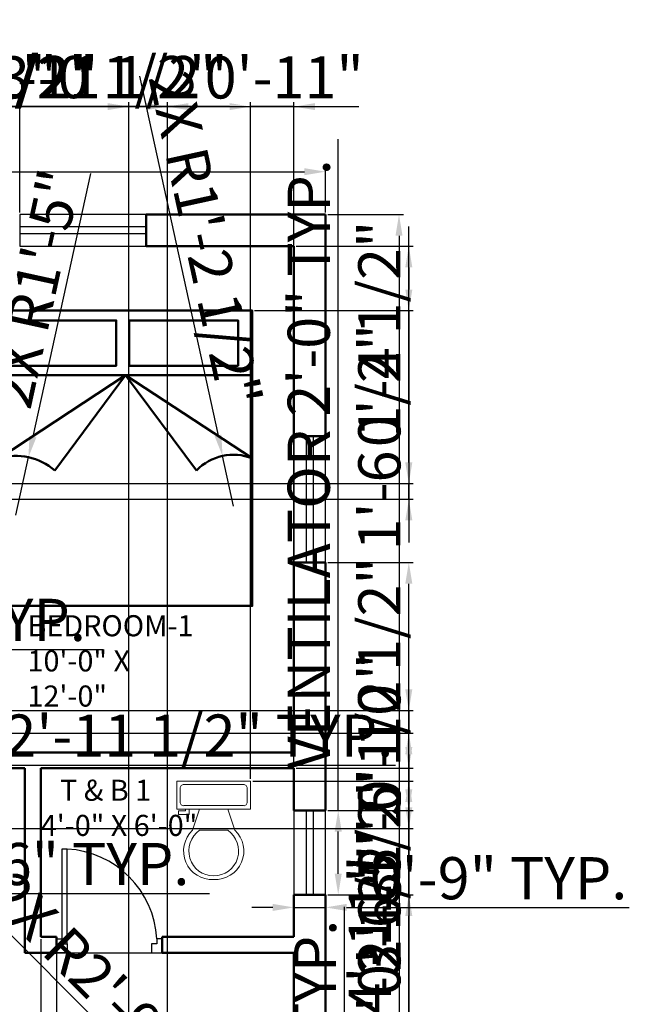
# Model space of a CAD drawing. Units: inches. Extents: x 1086 to 1501, y 383 to 973.
# Tile 7 of 7: x 1316 to 1490, y 611 to 891. Entities that reach past the tile are written whole.
import ezdxf

# ---------------------------------------------------------------- set-up
doc = ezdxf.new("R2010")
doc.units = ezdxf.units.IN
for name, color, linetype, lineweight in [('A-ANNO-DIMS', 2, 'Continuous', 18), ('A-AREA-IDEN', 7, 'Continuous', 25), ('A-FLOR-FIXT', 9, 'Continuous', 18), ('door', 10, 'Continuous', 25), ('furniture', 255, 'Continuous', 18), ('ventilator', 151, 'Continuous', 25), ('wall', 7, 'Continuous', 50), ('window', 81, 'Continuous', 25)]:
    doc.layers.add(name, color=color, linetype=linetype, lineweight=lineweight)
doc.styles.get("Standard").update_dxf_attribs({"font": 'arial.ttf'})
doc.dimstyles.new('ISO-25', dxfattribs={"dimtxt": 12, "dimasz": 6, "dimexe": 1.25, "dimexo": 0.625, "dimtad": 1, "dimdec": 1, "dimlunit": 3, "dimtxsty": 'Standard', "dimcen": 2.5, "dimadec": 0, "dimazin": 0, "dimtfac": 1, "dimtdec": 1, "dimtmove": 0, "dimatfit": 3, "dimfxl": 1, "dimarcsym": 0})

# ---------------------------------------------------------------- blocks, each defined once
blk = doc.blocks.new('d1')
at = {"layer": 'door'}
blk.add_line((1603.89, 536.69), (1633.89, 536.69), dxfattribs=at)
blk.add_lwpolyline([(1605.39, 539.19), (1606.89, 539.19), (1606.89, 566.19), (1605.39, 566.19)], close=True, dxfattribs=at)
for points in [[(1606.89, 536.69), (1603.89, 536.69), (1603.89, 540.69), (1605.39, 540.69), (1605.39, 539.19), (1606.89, 539.19), (1606.89, 536.69)], [(1630.89, 536.69), (1633.89, 536.69), (1633.89, 540.69), (1632.39, 540.69), (1632.39, 539.19), (1630.89, 539.19), (1630.89, 536.69)]]:
    blk.add_lwpolyline(points, dxfattribs=at)
blk.add_arc((1605.39, 539.19), 27.04, 3.1798, 86.8202, dxfattribs=at)
blk = doc.blocks.new('v')
at = {"layer": 'ventilator'}
for p, q in [((1539.56, 920.22), (1539.56, 896.22)), ((1541.56, 920.22), (1541.56, 896.22))]:
    blk.add_line(p, q, dxfattribs=at)
blk.add_lwpolyline([(1536.06, 896.22), (1545.06, 896.22), (1545.06, 920.22), (1536.06, 920.22)], close=True, dxfattribs=at)
blk = doc.blocks.new('w1')
at = {"layer": 'window'}
for p, q in [((1475.33, 845.32), (1475.33, 809.32)), ((1477.33, 845.32), (1477.33, 809.32))]:
    blk.add_line(p, q, dxfattribs=at)
blk.add_lwpolyline([(1471.83, 809.32), (1480.83, 809.32), (1480.83, 845.32), (1471.83, 845.32)], close=True, dxfattribs=at)
blk = doc.blocks.new('bed')
at = {"layer": 'wall'}
for p, q in [((1549.71, 859.44), (1621.71, 859.44)), ((1585.71, 859.44), (1549.71, 835.76)), ((1585.71, 859.44), (1565.54, 832.3)), ((1585.71, 859.44), (1621.71, 835.76)), ((1585.71, 859.44), (1605.88, 832.3))]:
    blk.add_line(p, q, dxfattribs=at)
for points in [[(1549.71, 793.76), (1621.71, 793.76), (1621.71, 877.76), (1549.71, 877.76)], [(1552.04, 875), (1583.04, 875), (1583.04, 862.08), (1552.04, 862.08)], [(1586.71, 875), (1617.71, 875), (1617.71, 862.08), (1586.71, 862.08)]]:
    blk.add_lwpolyline(points, close=True, dxfattribs=at)
for centre, radius, start, end in [((1554.45, 819.53), 16.91, 49.0428, 106.2967), ((1616.39, 822.13), 14.63, 68.7093, 135.9513)]:
    blk.add_arc(centre, radius, start, end, dxfattribs=at)
blk = doc.blocks.new('*U8')
for p, q in [((241.3, -152.4), (241.3, -50.8)), ((-203.2, -215.9), (-203.2, -203.2)), ((-177.8, -203.2), (-177.8, -241.3)), ((-101.6, -203.2), (-152.4, -355.6)), ((101.6, -203.2), (152.4, -355.6)), ((-254, -215.9), (-203.2, -215.9)), ((-254, -241.3), (-254, -215.9)), ((-177.8, -241.3), (-254, -241.3)), ((101.6, -355.6), (-101.6, -355.6))]:
    blk.add_line(p, q)
blk.add_lwpolyline([(266.7, -203.2), (266.7, 0), (-266.7, 0), (-266.7, -203.2)], close=True)
for points in [[(-241.3, -50.8), (-241.3, -152.4)], [(215.9, -25.4), (-215.9, -25.4)], [(-215.9, -177.8), (215.9, -177.8)]]:
    blk.add_lwpolyline(points)
for centre, radius, start, end in [((-219.075, -47.625), 22.45064, 81.8699, 188.1301), ((219.075, -47.625), 22.45064, 351.8699, 98.1301), ((-219.075, -155.575), 22.45064, 171.869898, 278.1301), ((219.075, -155.575), 22.45064, 261.8699, 8.1301), ((-12.12088, -505.93752), 205.61935, 133.01722, 273.38), ((0.94996, -504.77674), 181.02486, 124.50543, 269.7), ((-0.94742, -504.77674), 181.02486, 270.3, 55.4946), ((12.12342, -505.93752), 205.61935, 266.62, 46.9828)]:
    blk.add_arc(centre, radius, start, end)
blk = doc.blocks.new('*D9')
at = {"layer": 'A-ANNO-DIMS', "color": 0, "lineweight": -2, "transparency": 16777216}
for p, q in [((1133.43, 835.83), (1133.43, 848.67)), ((1139.43, 847.42), (1397.43, 847.42)), ((1403.43, 835.83), (1403.43, 848.67))]:
    blk.add_line(p, q, dxfattribs=at)
at = {"layer": 'A-ANNO-DIMS', "color": 0, "transparency": 16777216}
for points in [[(1139.43, 848.42), (1139.43, 846.42), (1133.43, 847.42)], [(1397.43, 848.42), (1397.43, 846.42), (1403.43, 847.42)]]:
    blk.add_solid(points, dxfattribs=at)
at = {"layer": 'Defpoints', "color": 0, "transparency": 16777216}
for p in [(1403.43, 847.42), (1133.43, 835.21), (1403.43, 835.21)]:
    blk.add_point(p, dxfattribs=at)
at = {"layer": 'A-ANNO-DIMS', "color": 0, "transparency": 16777216, "insert": (1268.43, 854.18), "char_height": 12, "attachment_point": 5}
blk.add_mtext('22\'-6"', dxfattribs=at)
blk = doc.blocks.new('*D10')
at = {"layer": 'A-ANNO-DIMS', "color": 0, "lineweight": -2, "transparency": 16777216}
for p, q in [((1404.05, 835.21), (1425.57, 835.21)), ((1424.32, 829.21), (1424.32, 422.21)), ((1404.05, 416.21), (1425.57, 416.21))]:
    blk.add_line(p, q, dxfattribs=at)
at = {"layer": 'A-ANNO-DIMS', "color": 0, "transparency": 16777216}
for points in [[(1423.32, 829.21), (1425.32, 829.21), (1424.32, 835.21)], [(1423.32, 422.21), (1425.32, 422.21), (1424.32, 416.21)]]:
    blk.add_solid(points, dxfattribs=at)
at = {"layer": 'Defpoints', "color": 0, "transparency": 16777216}
for p in [(1403.43, 835.21), (1403.43, 416.21), (1424.32, 416.21)]:
    blk.add_point(p, dxfattribs=at)
at = {"layer": 'A-ANNO-DIMS', "color": 0, "transparency": 16777216, "insert": (1417.56, 625.71), "char_height": 12, "attachment_point": 5, "rotation": 90}
blk.add_mtext('34\'-11"', dxfattribs=at)
blk = doc.blocks.new('*D13')
at = {"layer": 'A-ANNO-DIMS', "color": 0, "lineweight": -2, "transparency": 16777216}
for p, q in [((1408.83, 479.21), (1408.83, 638.31)), ((1404.05, 479.21), (1410.08, 479.21)), ((1408.83, 449.21), (1408.83, 473.21)), ((1404.05, 443.21), (1410.08, 443.21))]:
    blk.add_line(p, q, dxfattribs=at)
at = {"layer": 'A-ANNO-DIMS', "color": 0, "transparency": 16777216}
for points in [[(1407.83, 473.21), (1409.83, 473.21), (1408.83, 479.21)], [(1407.83, 449.21), (1409.83, 449.21), (1408.83, 443.21)]]:
    blk.add_solid(points, dxfattribs=at)
at = {"layer": 'Defpoints', "color": 0, "transparency": 16777216}
for p in [(1403.43, 479.21), (1408.83, 479.21), (1403.43, 443.21)]:
    blk.add_point(p, dxfattribs=at)
at = {"layer": 'A-ANNO-DIMS', "color": 0, "transparency": 16777216, "insert": (1401.99, 561.76), "char_height": 12, "attachment_point": 5, "rotation": 90}
blk.add_mtext('WINDOW 3\'-0" TYP.', dxfattribs=at)
blk = doc.blocks.new('*D15')
at = {"layer": 'A-ANNO-DIMS', "color": 0, "lineweight": -2, "transparency": 16777216}
for p, q in [((1407.03, 665.71), (1407.03, 856.64)), ((1404.05, 665.71), (1408.28, 665.71)), ((1407.03, 647.71), (1407.03, 659.71)), ((1404.05, 641.71), (1408.28, 641.71))]:
    blk.add_line(p, q, dxfattribs=at)
at = {"layer": 'A-ANNO-DIMS', "color": 0, "transparency": 16777216}
for points in [[(1406.03, 659.71), (1408.03, 659.71), (1407.03, 665.71)], [(1406.03, 647.71), (1408.03, 647.71), (1407.03, 641.71)]]:
    blk.add_solid(points, dxfattribs=at)
at = {"layer": 'Defpoints', "color": 0, "transparency": 16777216}
for p in [(1403.43, 665.71), (1407.03, 665.71), (1403.43, 641.71)]:
    blk.add_point(p, dxfattribs=at)
at = {"layer": 'A-ANNO-DIMS', "color": 0, "transparency": 16777216, "insert": (1400.2, 764.17), "char_height": 12, "attachment_point": 5, "rotation": 90}
blk.add_mtext('VENTILATOR 2\'-0" TYP.', dxfattribs=at)
blk = doc.blocks.new('*D16')
at = {"layer": 'A-ANNO-DIMS', "color": 0, "lineweight": -2, "transparency": 16777216}
for p, q in [((1394.43, 641.08), (1394.43, 636.86)), ((1403.43, 641.08), (1403.43, 636.86)), ((1388.43, 638.11), (1382.43, 638.11)), ((1394.43, 638.11), (1403.43, 638.11)), ((1409.43, 638.11), (1489.83, 638.11))]:
    blk.add_line(p, q, dxfattribs=at)
at = {"layer": 'A-ANNO-DIMS', "color": 0, "transparency": 16777216}
for points in [[(1388.43, 639.11), (1388.43, 637.11), (1394.43, 638.11)], [(1409.43, 639.11), (1409.43, 637.11), (1403.43, 638.11)]]:
    blk.add_solid(points, dxfattribs=at)
at = {"layer": 'Defpoints', "color": 0, "transparency": 16777216}
for p in [(1394.43, 641.71), (1403.43, 641.71), (1403.43, 638.11)]:
    blk.add_point(p, dxfattribs=at)
at = {"layer": 'A-ANNO-DIMS', "color": 0, "transparency": 16777216, "insert": (1452.63, 644.86), "char_height": 12, "attachment_point": 5}
blk.add_mtext('0\'-9" TYP.', dxfattribs=at)
blk = doc.blocks.new('*D19')
at = {"layer": 'A-ANNO-DIMS', "color": 0, "lineweight": -2, "transparency": 16777216}
for p, q in [((1306.05, 673.21), (1312.08, 673.21)), ((1310.83, 667.21), (1310.83, 643.21)), ((1306.05, 637.21), (1312.08, 637.21)), ((1310.83, 637.21), (1310.83, 411.12))]:
    blk.add_line(p, q, dxfattribs=at)
at = {"layer": 'A-ANNO-DIMS', "color": 0, "transparency": 16777216}
for points in [[(1309.83, 667.21), (1311.83, 667.21), (1310.83, 673.21)], [(1309.83, 643.21), (1311.83, 643.21), (1310.83, 637.21)]]:
    blk.add_solid(points, dxfattribs=at)
at = {"layer": 'Defpoints', "color": 0, "transparency": 16777216}
for p in [(1305.43, 673.21), (1305.43, 637.21), (1310.83, 637.21)]:
    blk.add_point(p, dxfattribs=at)
at = {"layer": 'A-ANNO-DIMS', "color": 0, "transparency": 16777216, "insert": (1303.99, 521.16), "char_height": 12, "attachment_point": 5, "rotation": 90}
blk.add_mtext('BEDROOM DOOR 3\'-0" TYP.', dxfattribs=at)
blk = doc.blocks.new('*D20')
at = {"layer": 'A-ANNO-DIMS', "color": 0, "lineweight": -2, "transparency": 16777216}
for p, q in [((1269.93, 673.83), (1269.93, 679.86)), ((1275.93, 678.61), (1299.43, 678.61)), ((1305.43, 673.83), (1305.43, 679.86)), ((1305.43, 678.61), (1423.32, 678.61))]:
    blk.add_line(p, q, dxfattribs=at)
at = {"layer": 'A-ANNO-DIMS', "color": 0, "transparency": 16777216}
for points in [[(1275.93, 679.61), (1275.93, 677.61), (1269.93, 678.61)], [(1299.43, 679.61), (1299.43, 677.61), (1305.43, 678.61)]]:
    blk.add_solid(points, dxfattribs=at)
at = {"layer": 'Defpoints', "color": 0, "transparency": 16777216}
for p in [(1305.43, 678.61), (1269.93, 673.21), (1305.43, 673.21)]:
    blk.add_point(p, dxfattribs=at)
at = {"layer": 'A-ANNO-DIMS', "color": 0, "transparency": 16777216, "insert": (1367.37, 685.44), "char_height": 12, "attachment_point": 5}
blk.add_mtext('2\'-11 1/2" TYP.', dxfattribs=at)
blk = doc.blocks.new('*D25')
at = {"layer": 'A-ANNO-DIMS', "color": 0, "lineweight": -2, "transparency": 16777216}
for p, q in [((1147.7, 709.78), (1147.7, 712.78)), ((1153.7, 711.53), (1157.51, 711.53)), ((1163.51, 709.78), (1163.51, 712.78)), ((1163.51, 711.53), (1340.15, 711.53))]:
    blk.add_line(p, q, dxfattribs=at)
at = {"layer": 'A-ANNO-DIMS', "color": 0, "transparency": 16777216}
for points in [[(1153.7, 712.53), (1153.7, 710.53), (1147.7, 711.53)], [(1157.51, 712.53), (1157.51, 710.53), (1163.51, 711.53)]]:
    blk.add_solid(points, dxfattribs=at)
at = {"layer": 'Defpoints', "color": 0, "transparency": 16777216}
for p in [(1163.51, 711.53), (1147.7, 709.16), (1163.51, 709.16)]:
    blk.add_point(p, dxfattribs=at)
at = {"layer": 'A-ANNO-DIMS', "color": 0, "transparency": 16777216, "insert": (1254.83, 718.36), "char_height": 12, "attachment_point": 5}
blk.add_mtext('END CHAIR 1\'-4" TYP.', dxfattribs=at)
blk = doc.blocks.new('*D27')
at = {"layer": 'A-ANNO-DIMS', "color": 0, "lineweight": -2, "transparency": 16777216}
for p, q in [((1171.32, 644.17), (1171.32, 640.82)), ((1177.32, 642.07), (1183.45, 642.07)), ((1189.45, 644.17), (1189.45, 640.82)), ((1189.45, 642.07), (1370.39, 642.07))]:
    blk.add_line(p, q, dxfattribs=at)
at = {"layer": 'A-ANNO-DIMS', "color": 0, "transparency": 16777216}
for points in [[(1177.32, 643.07), (1177.32, 641.07), (1171.32, 642.07)], [(1183.45, 643.07), (1183.45, 641.07), (1189.45, 642.07)]]:
    blk.add_solid(points, dxfattribs=at)
at = {"layer": 'Defpoints', "color": 0, "transparency": 16777216}
for p in [(1171.32, 644.79), (1189.45, 644.79), (1189.45, 642.07)]:
    blk.add_point(p, dxfattribs=at)
at = {"layer": 'A-ANNO-DIMS', "color": 0, "transparency": 16777216, "insert": (1282.92, 648.9), "char_height": 12, "attachment_point": 5}
blk.add_mtext('SIDE CHAIR 1\'-6" TYP.', dxfattribs=at)
blk = doc.blocks.new('*D31')
at = {"layer": 'A-ANNO-DIMS', "color": 0, "lineweight": -2, "transparency": 16777216}
for p, q in [((1256.43, 835.83), (1256.43, 867.19)), ((1262.43, 865.94), (1310.43, 865.94)), ((1316.43, 835.83), (1316.43, 867.19))]:
    blk.add_line(p, q, dxfattribs=at)
at = {"layer": 'A-ANNO-DIMS', "color": 0, "transparency": 16777216}
for points in [[(1262.43, 866.94), (1262.43, 864.94), (1256.43, 865.94)], [(1310.43, 866.94), (1310.43, 864.94), (1316.43, 865.94)]]:
    blk.add_solid(points, dxfattribs=at)
at = {"layer": 'Defpoints', "color": 0, "transparency": 16777216}
for p in [(1316.43, 865.94), (1256.43, 835.21), (1316.43, 835.21)]:
    blk.add_point(p, dxfattribs=at)
at = {"layer": 'A-ANNO-DIMS', "color": 0, "transparency": 16777216, "insert": (1286.43, 872.69), "char_height": 12, "attachment_point": 5}
blk.add_mtext('5\'-0"', dxfattribs=at)
blk = doc.blocks.new('*D36')
at = {"layer": 'A-ANNO-DIMS', "color": 0, "lineweight": -2, "transparency": 16777216}
for p, q in [((1427.11, 641.71), (1427.11, 708.82)), ((1404.05, 641.71), (1428.36, 641.71)), ((1427.11, 587.46), (1427.11, 635.71)), ((1404.05, 581.46), (1428.36, 581.46))]:
    blk.add_line(p, q, dxfattribs=at)
at = {"layer": 'A-ANNO-DIMS', "color": 0, "transparency": 16777216}
for points in [[(1426.11, 635.71), (1428.11, 635.71), (1427.11, 641.71)], [(1426.11, 587.46), (1428.11, 587.46), (1427.11, 581.46)]]:
    blk.add_solid(points, dxfattribs=at)
at = {"layer": 'Defpoints', "color": 0, "transparency": 16777216}
for p in [(1403.43, 641.71), (1427.11, 641.71), (1403.43, 581.46)]:
    blk.add_point(p, dxfattribs=at)
at = {"layer": 'A-ANNO-DIMS', "color": 0, "transparency": 16777216, "insert": (1420.28, 678.26), "char_height": 12, "attachment_point": 5, "rotation": 90}
blk.add_mtext('5\'-0 1/2"', dxfattribs=at)
blk = doc.blocks.new('*D37')
at = {"layer": 'A-ANNO-DIMS', "color": 0, "lineweight": -2, "transparency": 16777216}
for p, q in [((1404.05, 736.21), (1428.36, 736.21)), ((1427.11, 671.71), (1427.11, 730.21)), ((1404.05, 665.71), (1428.36, 665.71))]:
    blk.add_line(p, q, dxfattribs=at)
at = {"layer": 'A-ANNO-DIMS', "color": 0, "transparency": 16777216}
for points in [[(1426.11, 730.21), (1428.11, 730.21), (1427.11, 736.21)], [(1426.11, 671.71), (1428.11, 671.71), (1427.11, 665.71)]]:
    blk.add_solid(points, dxfattribs=at)
at = {"layer": 'Defpoints', "color": 0, "transparency": 16777216}
for p in [(1403.43, 736.21), (1427.11, 736.21), (1403.43, 665.71)]:
    blk.add_point(p, dxfattribs=at)
at = {"layer": 'A-ANNO-DIMS', "color": 0, "transparency": 16777216, "insert": (1420.28, 700.96), "char_height": 12, "attachment_point": 5, "rotation": 90}
blk.add_mtext('5\'-10 1/2"', dxfattribs=at)
blk = doc.blocks.new('*D42')
at = {"layer": 'A-ANNO-DIMS', "color": 0, "lineweight": -2, "transparency": 16777216}
for p, q in [((1256.43, 502.33), (1256.43, 867.19)), ((1262.43, 865.94), (1263.93, 865.94)), ((1269.93, 502.33), (1269.93, 867.19)), ((1269.93, 865.94), (1335.91, 865.94))]:
    blk.add_line(p, q, dxfattribs=at)
at = {"layer": 'A-ANNO-DIMS', "color": 0, "transparency": 16777216}
for points in [[(1262.43, 866.94), (1262.43, 864.94), (1256.43, 865.94)], [(1263.93, 866.94), (1263.93, 864.94), (1269.93, 865.94)]]:
    blk.add_solid(points, dxfattribs=at)
at = {"layer": 'Defpoints', "color": 0, "transparency": 16777216}
for p in [(1269.93, 865.94), (1256.43, 501.71), (1269.93, 501.71)]:
    blk.add_point(p, dxfattribs=at)
at = {"layer": 'A-ANNO-DIMS', "color": 0, "transparency": 16777216, "insert": (1305.92, 872.77), "char_height": 12, "attachment_point": 5}
blk.add_mtext('1\'-1 1/2"', dxfattribs=at)
blk = doc.blocks.new('*D45')
at = {"layer": 'A-ANNO-DIMS', "color": 0, "lineweight": -2, "transparency": 16777216}
for p, q in [((1259.43, 497.83), (1259.43, 867.19)), ((1265.43, 865.94), (1352.43, 865.94)), ((1358.43, 497.83), (1358.43, 867.19))]:
    blk.add_line(p, q, dxfattribs=at)
at = {"layer": 'A-ANNO-DIMS', "color": 0, "transparency": 16777216}
for points in [[(1265.43, 866.94), (1265.43, 864.94), (1259.43, 865.94)], [(1352.43, 866.94), (1352.43, 864.94), (1358.43, 865.94)]]:
    blk.add_solid(points, dxfattribs=at)
at = {"layer": 'Defpoints', "color": 0, "transparency": 16777216}
for p in [(1358.43, 865.94), (1259.43, 497.21), (1358.43, 497.21)]:
    blk.add_point(p, dxfattribs=at)
at = {"layer": 'A-ANNO-DIMS', "color": 0, "transparency": 16777216, "insert": (1308.93, 872.7), "char_height": 12, "attachment_point": 5}
blk.add_mtext('8\'-3"', dxfattribs=at)
blk = doc.blocks.new('*D47')
at = {"layer": 'A-ANNO-DIMS', "color": 0, "lineweight": -2, "transparency": 16777216}
for p, q in [((1341.43, 865.94), (1335.43, 865.94)), ((1347.43, 425.83), (1347.43, 867.19)), ((1347.43, 865.94), (1358.43, 865.94)), ((1358.43, 425.83), (1358.43, 867.19)), ((1364.43, 865.94), (1412.9, 865.94))]:
    blk.add_line(p, q, dxfattribs=at)
at = {"layer": 'A-ANNO-DIMS', "color": 0, "transparency": 16777216}
for points in [[(1341.43, 866.94), (1341.43, 864.94), (1347.43, 865.94)], [(1364.43, 866.94), (1364.43, 864.94), (1358.43, 865.94)]]:
    blk.add_solid(points, dxfattribs=at)
at = {"layer": 'Defpoints', "color": 0, "transparency": 16777216}
for p in [(1358.43, 865.94), (1347.43, 425.21), (1358.43, 425.21)]:
    blk.add_point(p, dxfattribs=at)
at = {"layer": 'A-ANNO-DIMS', "color": 0, "transparency": 16777216, "insert": (1391.67, 872.69), "char_height": 12, "attachment_point": 5}
blk.add_mtext('0\'-11"', dxfattribs=at)
blk = doc.blocks.new('*D54')
at = {"layer": 'A-ANNO-DIMS', "color": 0, "lineweight": -2, "transparency": 16777216}
for p, q in [((1427.11, 764.71), (1427.11, 831.82)), ((1270.55, 758.71), (1428.36, 758.71)), ((1427.11, 754.21), (1427.11, 758.71)), ((1270.55, 754.21), (1428.36, 754.21)), ((1427.11, 748.21), (1427.11, 742.21))]:
    blk.add_line(p, q, dxfattribs=at)
at = {"layer": 'A-ANNO-DIMS', "color": 0, "transparency": 16777216}
for points in [[(1426.11, 764.71), (1428.11, 764.71), (1427.11, 758.71)], [(1426.11, 748.21), (1428.11, 748.21), (1427.11, 754.21)]]:
    blk.add_solid(points, dxfattribs=at)
at = {"layer": 'Defpoints', "color": 0, "transparency": 16777216}
for p in [(1269.93, 758.71), (1427.11, 758.71), (1269.93, 754.21)]:
    blk.add_point(p, dxfattribs=at)
at = {"layer": 'A-ANNO-DIMS', "color": 0, "transparency": 16777216, "insert": (1420.28, 801.26), "char_height": 12, "attachment_point": 5, "rotation": 90}
blk.add_mtext('0\'-4 1/2"', dxfattribs=at)
blk = doc.blocks.new('*D60')
at = {"layer": 'A-ANNO-DIMS', "color": 0, "lineweight": -2, "transparency": 16777216}
for p, q in [((1322.43, 629.08), (1322.43, 392.46)), ((1326.93, 629.08), (1326.93, 392.46)), ((1316.43, 393.71), (1310.43, 393.71)), ((1322.43, 393.71), (1326.93, 393.71)), ((1332.93, 393.71), (1400.04, 393.71))]:
    blk.add_line(p, q, dxfattribs=at)
at = {"layer": 'A-ANNO-DIMS', "color": 0, "transparency": 16777216}
for points in [[(1316.43, 394.71), (1316.43, 392.71), (1322.43, 393.71)], [(1332.93, 394.71), (1332.93, 392.71), (1326.93, 393.71)]]:
    blk.add_solid(points, dxfattribs=at)
at = {"layer": 'Defpoints', "color": 0, "transparency": 16777216}
for p in [(1322.43, 629.71), (1326.93, 629.71), (1326.93, 393.71)]:
    blk.add_point(p, dxfattribs=at)
at = {"layer": 'A-ANNO-DIMS', "color": 0, "transparency": 16777216, "insert": (1369.49, 400.54), "char_height": 12, "attachment_point": 5}
blk.add_mtext('0\'-4 1/2"', dxfattribs=at)
blk = doc.blocks.new('*D61')
at = {"layer": 'A-ANNO-DIMS', "color": 0, "lineweight": -2, "transparency": 16777216}
for p, q in [((1376.11, 865.94), (1310.13, 865.94)), ((1382.11, 674.69), (1382.11, 867.19)), ((1394.43, 865.94), (1382.11, 865.94)), ((1394.43, 678.33), (1394.43, 867.19)), ((1400.43, 865.94), (1406.43, 865.94))]:
    blk.add_line(p, q, dxfattribs=at)
at = {"layer": 'A-ANNO-DIMS', "color": 0, "transparency": 16777216}
for points in [[(1376.11, 866.94), (1376.11, 864.94), (1382.11, 865.94)], [(1400.43, 866.94), (1400.43, 864.94), (1394.43, 865.94)]]:
    blk.add_solid(points, dxfattribs=at)
at = {"layer": 'Defpoints', "color": 0, "transparency": 16777216}
for p in [(1382.11, 865.94), (1394.43, 677.71), (1382.11, 674.06)]:
    blk.add_point(p, dxfattribs=at)
at = {"layer": 'A-ANNO-DIMS', "color": 0, "transparency": 16777216, "insert": (1340.12, 872.77), "char_height": 12, "attachment_point": 5}
blk.add_mtext('1\'-0 1/2"', dxfattribs=at)
blk = doc.blocks.new('*D62')
at = {"layer": 'A-ANNO-DIMS', "color": 0, "lineweight": -2, "transparency": 16777216}
for p, q in [((1427.11, 683.71), (1427.11, 689.71)), ((1395.05, 677.71), (1428.36, 677.71)), ((1427.11, 677.71), (1427.11, 674.06)), ((1382.74, 674.06), (1428.36, 674.06)), ((1427.11, 668.06), (1427.11, 600.95))]:
    blk.add_line(p, q, dxfattribs=at)
at = {"layer": 'A-ANNO-DIMS', "color": 0, "transparency": 16777216}
for points in [[(1426.11, 683.71), (1428.11, 683.71), (1427.11, 677.71)], [(1426.11, 668.06), (1428.11, 668.06), (1427.11, 674.06)]]:
    blk.add_solid(points, dxfattribs=at)
at = {"layer": 'Defpoints', "color": 0, "transparency": 16777216}
for p in [(1394.43, 677.71), (1382.11, 674.06), (1427.11, 674.06)]:
    blk.add_point(p, dxfattribs=at)
at = {"layer": 'A-ANNO-DIMS', "color": 0, "transparency": 16777216, "insert": (1420.28, 631.51), "char_height": 12, "attachment_point": 5, "rotation": 90}
blk.add_mtext('0\'-3 1/2"', dxfattribs=at)
blk = doc.blocks.new('*D66')
at = {"layer": 'A-ANNO-DIMS', "color": 0, "lineweight": -2, "transparency": 16777216}
for p, q in [((1190.08, 687.66), (1428.36, 687.66)), ((1427.11, 681.66), (1427.11, 666.6)), ((1190.08, 660.6), (1428.36, 660.6)), ((1427.11, 660.6), (1427.11, 621.25))]:
    blk.add_line(p, q, dxfattribs=at)
at = {"layer": 'A-ANNO-DIMS', "color": 0, "transparency": 16777216}
for points in [[(1426.11, 681.66), (1428.11, 681.66), (1427.11, 687.66)], [(1426.11, 666.6), (1428.11, 666.6), (1427.11, 660.6)]]:
    blk.add_solid(points, dxfattribs=at)
at = {"layer": 'Defpoints', "color": 0, "transparency": 16777216}
for p in [(1189.45, 687.66), (1189.45, 660.6), (1427.11, 660.6)]:
    blk.add_point(p, dxfattribs=at)
at = {"layer": 'A-ANNO-DIMS', "color": 0, "transparency": 16777216, "insert": (1420.36, 637.93), "char_height": 12, "attachment_point": 5, "rotation": 90}
blk.add_mtext('2\'-3"', dxfattribs=at)
blk = doc.blocks.new('*D67')
at = {"layer": 'A-ANNO-DIMS', "color": 0, "lineweight": -2, "transparency": 16777216}
for p, q in [((1427.11, 700.13), (1427.11, 706.13)), ((1171.95, 694.13), (1428.36, 694.13)), ((1427.11, 694.13), (1427.11, 687.66)), ((1190.08, 687.66), (1428.36, 687.66)), ((1427.11, 681.66), (1427.11, 614.55))]:
    blk.add_line(p, q, dxfattribs=at)
at = {"layer": 'A-ANNO-DIMS', "color": 0, "transparency": 16777216}
for points in [[(1426.11, 700.13), (1428.11, 700.13), (1427.11, 694.13)], [(1426.11, 681.66), (1428.11, 681.66), (1427.11, 687.66)]]:
    blk.add_solid(points, dxfattribs=at)
at = {"layer": 'Defpoints', "color": 0, "transparency": 16777216}
for p in [(1171.32, 694.13), (1189.45, 687.66), (1427.11, 687.66)]:
    blk.add_point(p, dxfattribs=at)
at = {"layer": 'A-ANNO-DIMS', "color": 0, "transparency": 16777216, "insert": (1420.28, 645.1), "char_height": 12, "attachment_point": 5, "rotation": 90}
blk.add_mtext('0\'-6 1/2"', dxfattribs=at)
blk = doc.blocks.new('*D69')
at = {"layer": 'A-ANNO-DIMS', "color": 0, "lineweight": -2, "transparency": 16777216}
for p, q in [((1236.63, 603.21), (1236.63, 867.19)), ((1242.63, 865.94), (1263.93, 865.94)), ((1269.93, 603.25), (1269.93, 867.19)), ((1269.93, 865.94), (1337.25, 865.94))]:
    blk.add_line(p, q, dxfattribs=at)
at = {"layer": 'A-ANNO-DIMS', "color": 0, "transparency": 16777216}
for points in [[(1242.63, 866.94), (1242.63, 864.94), (1236.63, 865.94)], [(1263.93, 866.94), (1263.93, 864.94), (1269.93, 865.94)]]:
    blk.add_solid(points, dxfattribs=at)
at = {"layer": 'Defpoints', "color": 0, "transparency": 16777216}
for p in [(1269.93, 865.94), (1236.63, 602.59), (1269.93, 602.62)]:
    blk.add_point(p, dxfattribs=at)
at = {"layer": 'A-ANNO-DIMS', "color": 0, "transparency": 16777216, "insert": (1306.59, 872.77), "char_height": 12, "attachment_point": 5}
blk.add_mtext('2\'-9 1/2"', dxfattribs=at)
blk = doc.blocks.new('*D74')
at = {"layer": 'A-ANNO-DIMS', "color": 0, "lineweight": -2, "transparency": 16777216}
for p, q in [((1395.05, 826.21), (1428.36, 826.21)), ((1427.11, 820.21), (1427.11, 813.89)), ((1383.18, 807.89), (1428.36, 807.89)), ((1427.11, 807.89), (1427.11, 741.91))]:
    blk.add_line(p, q, dxfattribs=at)
at = {"layer": 'A-ANNO-DIMS', "color": 0, "transparency": 16777216}
for points in [[(1426.11, 820.21), (1428.11, 820.21), (1427.11, 826.21)], [(1426.11, 813.89), (1428.11, 813.89), (1427.11, 807.89)]]:
    blk.add_solid(points, dxfattribs=at)
at = {"layer": 'Defpoints', "color": 0, "transparency": 16777216}
for p in [(1394.43, 826.21), (1382.55, 807.89), (1427.11, 807.89)]:
    blk.add_point(p, dxfattribs=at)
at = {"layer": 'A-ANNO-DIMS', "color": 0, "transparency": 16777216, "insert": (1420.28, 771.9), "char_height": 12, "attachment_point": 5, "rotation": 90}
blk.add_mtext('1\'-6 1/2"', dxfattribs=at)
blk = doc.blocks.new('*D77')
at = {"layer": 'A-ANNO-DIMS', "color": 0, "lineweight": -2, "transparency": 16777216}
for p, q in [((1274.43, 502.33), (1274.43, 867.19)), ((1280.43, 865.94), (1292.14, 865.94)), ((1298.14, 513.04), (1298.14, 867.19)), ((1298.14, 865.94), (1373.44, 865.94))]:
    blk.add_line(p, q, dxfattribs=at)
at = {"layer": 'A-ANNO-DIMS', "color": 0, "transparency": 16777216}
for points in [[(1280.43, 866.94), (1280.43, 864.94), (1274.43, 865.94)], [(1292.14, 866.94), (1292.14, 864.94), (1298.14, 865.94)]]:
    blk.add_solid(points, dxfattribs=at)
at = {"layer": 'Defpoints', "color": 0, "transparency": 16777216}
for p in [(1298.14, 865.94), (1298.14, 512.42), (1274.43, 501.71)]:
    blk.add_point(p, dxfattribs=at)
at = {"layer": 'A-ANNO-DIMS', "color": 0, "transparency": 16777216, "insert": (1338.79, 872.77), "char_height": 12, "attachment_point": 5}
blk.add_mtext('1\'-11 1/2"', dxfattribs=at)
blk = doc.blocks.new('*D78')
at = {"layer": 'A-ANNO-DIMS', "color": 0, "lineweight": -2, "transparency": 16777216}
for p, q in [((1272.43, 671.71), (1295.79, 648.35)), ((1354.21, 589.92), (1300.03, 644.11))]:
    blk.add_line(p, q, dxfattribs=at)
at = {"layer": 'A-ANNO-DIMS', "color": 0, "transparency": 16777216}
blk.add_solid([(1300.74, 644.81), (1299.32, 643.4), (1295.79, 648.35)], dxfattribs=at)
at = {"layer": 'Defpoints', "color": 0, "transparency": 16777216}
for p in [(1272.43, 671.71), (1295.79, 648.35)]:
    blk.add_point(p, dxfattribs=at)
at = {"layer": 'A-ANNO-DIMS', "color": 0, "transparency": 16777216, "insert": (1334.02, 619.67), "char_height": 12, "attachment_point": 5, "rotation": 314.9994}
blk.add_mtext('2X R2\'-9"', dxfattribs=at)
blk = doc.blocks.new('*D81')
at = {"layer": 'A-ANNO-DIMS', "color": 0, "lineweight": -2, "transparency": 16777216}
for p, q in [((1336.56, 846.9), (1320.19, 772.04)), ((1315.3, 749.66), (1318.91, 766.18))]:
    blk.add_line(p, q, dxfattribs=at)
at = {"layer": 'A-ANNO-DIMS', "color": 0, "transparency": 16777216}
blk.add_solid([(1319.22, 772.25), (1321.17, 771.83), (1318.91, 766.18)], dxfattribs=at)
at = {"layer": 'Defpoints', "color": 0, "transparency": 16777216}
for p in [(1318.91, 766.18), (1315.3, 749.66)]:
    blk.add_point(p, dxfattribs=at)
at = {"layer": 'A-ANNO-DIMS', "color": 0, "transparency": 16777216, "insert": (1322.42, 813.84), "char_height": 12, "attachment_point": 5, "rotation": 77.6694}
blk.add_mtext('2X R1\'-5"', dxfattribs=at)
blk = doc.blocks.new('*D82')
at = {"layer": 'A-ANNO-DIMS', "color": 0, "lineweight": -2, "transparency": 16777216}
for p, q in [((1350.51, 874.58), (1372.84, 772.41)), ((1377.24, 752.26), (1374.12, 766.55))]:
    blk.add_line(p, q, dxfattribs=at)
at = {"layer": 'A-ANNO-DIMS', "color": 0, "transparency": 16777216}
blk.add_solid([(1373.81, 772.63), (1371.86, 772.2), (1374.12, 766.55)], dxfattribs=at)
at = {"layer": 'Defpoints', "color": 0, "transparency": 16777216}
for p in [(1374.12, 766.55), (1377.24, 752.26)]:
    blk.add_point(p, dxfattribs=at)
at = {"layer": 'A-ANNO-DIMS', "color": 0, "transparency": 16777216, "insert": (1367.7, 827.89), "char_height": 12, "attachment_point": 5, "rotation": 282.3285}
blk.add_mtext('2X R1\'-2 1/2"', dxfattribs=at)

msp = doc.modelspace()

# ---------------------------------------------------------------- linework, layer by layer
at = {"layer": 'wall'}
for p, q in [((1403.43, 835.21), (1352.43, 835.21)), ((1352.43, 826.21), (1352.43, 835.21)), ((1403.43, 772.21), (1403.43, 835.21)), ((1394.43, 826.21), (1352.43, 826.21)), ((1394.43, 772.21), (1394.43, 826.21)), ((1394.43, 772.21), (1403.43, 772.21)), ((1394.43, 682.21), (1394.43, 736.21)), ((1394.43, 736.21), (1403.43, 736.21)), ((1403.43, 665.71), (1403.43, 736.21)), ((1394.43, 682.21), (1274.43, 682.21)), ((1317.93, 677.71), (1274.43, 677.71)), ((1317.93, 625.21), (1317.93, 677.71)), ((1394.43, 677.71), (1322.43, 677.71)), ((1322.43, 629.71), (1322.43, 677.71)), ((1394.43, 665.71), (1394.43, 677.71)), ((1394.43, 665.71), (1403.43, 665.71)), ((1394.43, 629.71), (1394.43, 641.71)), ((1394.43, 641.71), (1403.43, 641.71)), ((1403.43, 581.46), (1403.43, 641.71)), ((1326.93, 629.71), (1322.43, 629.71)), ((1326.93, 625.21), (1326.93, 629.71)), ((1394.43, 629.71), (1356.93, 629.71)), ((1356.93, 625.21), (1356.93, 629.71)), ((1326.93, 625.21), (1317.93, 625.21)), ((1394.43, 625.21), (1356.93, 625.21)), ((1394.43, 581.46), (1394.43, 625.21))]:
    msp.add_line(p, q, dxfattribs=at)

# ---------------------------------------------------------------- block references
at = {"layer": 'A-FLOR-FIXT', "xscale": 0.0393700787401575, "yscale": 0.0393700787401575, "zscale": 0.0393700787401575}
msp.add_blockref('*U8', (1371.61, 674.06), dxfattribs=at)
at = {"layer": 'door'}
msp.add_blockref('d1', (-276.96, 88.52), dxfattribs=at)
at = {"layer": 'furniture'}
msp.add_blockref('bed', (-239.15, -69.87), dxfattribs=at)
at = {"layer": 'ventilator'}
msp.add_blockref('v', (-141.63, -254.51), dxfattribs=at)
at = {"layer": 'window', "rotation": 270}
msp.add_blockref('w1', (507.11, 2307.04), dxfattribs=at)
at = {"layer": 'window'}
msp.add_blockref('w1', (-77.4, -73.11), dxfattribs=at)

# ---------------------------------------------------------------- texts
at = {"layer": 'A-AREA-IDEN', "char_height": 6, "attachment_point": 1}
for s, insert in [('BEDROOM-1\\P10\'-0" X 12\'-0"', (1318.65, 721.25)), ('   T & B 1\\P4\'-0" X 6\'-0"', (1322.43, 674.45))]:
    msp.add_mtext_dynamic_manual_height_columns(s, width=53.2651, gutter_width=12.5, heights=[0], dxfattribs=dict(at, insert=insert))

# ---------------------------------------------------------------- dimensions: what is measured, and where the dimension line sits
at = {"layer": 'A-ANNO-DIMS'}
for base, p1, p2, override, picture, middle in [((1269.93, 865.94), (1236.63, 602.59), (1269.93, 602.62), {"dimdec": 1, "dimlfac": 1, "dimrnd": 0, "dimzin": 1, "dimdsep": 46, "dimlunit": 4, "dimfrac": 2}, '*D69', (1306.59, 872.77)), ((1269.93, 865.94), (1256.43, 501.71), (1269.93, 501.71), {"dimdec": 1, "dimlfac": 1, "dimrnd": 0, "dimzin": 1, "dimdsep": 46, "dimlunit": 4, "dimfrac": 2}, '*D42', (1305.92, 872.77)), ((1298.14, 865.94), (1274.43, 501.71), (1298.14, 512.42), {"dimdec": 1, "dimlfac": 1, "dimrnd": 0, "dimzin": 1, "dimdsep": 46, "dimlunit": 4, "dimfrac": 2}, '*D77', (1338.79, 872.77)), ((1382.11, 865.94), (1394.43, 677.71), (1382.11, 674.06), {"dimdec": 1, "dimlfac": 1, "dimrnd": 0, "dimzin": 1, "dimdsep": 46, "dimlunit": 4, "dimfrac": 2}, '*D61', (1340.12, 872.77)), ((1316.43, 865.94), (1256.43, 835.21), (1316.43, 835.21), {"dimdec": 1, "dimlfac": 1, "dimrnd": 0, "dimzin": 1, "dimdsep": 46, "dimlunit": 4, "dimfrac": 2}, '*D31', (1286.43, 872.69)), ((1358.43, 865.94), (1259.43, 497.21), (1358.43, 497.21), {"dimdec": 1, "dimlfac": 1, "dimrnd": 0, "dimzin": 1, "dimdsep": 46, "dimlunit": 4, "dimfrac": 2}, '*D45', (1308.93, 872.7)), ((1358.43, 865.94), (1347.43, 425.21), (1358.43, 425.21), {"dimdec": 1, "dimlfac": 1, "dimrnd": 0, "dimzin": 1, "dimdsep": 46, "dimlunit": 4, "dimfrac": 2}, '*D47', (1391.67, 872.69)), ((1403.43, 847.42), (1133.43, 835.21), (1403.43, 835.21), {"dimclrd": 0, "dimclre": 0, "dimclrt": 0}, '*D9', (1268.43, 854.18)), ((1326.93, 393.71), (1322.43, 629.71), (1326.93, 629.71), {"dimdec": 1, "dimlfac": 1, "dimrnd": 0, "dimzin": 1, "dimdsep": 46, "dimlunit": 4, "dimfrac": 2}, '*D60', (1369.49, 400.54))]:
    dim = msp.add_linear_dim(base=base, p1=p1, p2=p2, dimstyle='ISO-25', override=override, dxfattribs=at)
    dim.commit()
    dim.dimension.update_dxf_attribs({"geometry": picture, "text_midpoint": middle})
for center, mpoint, picture, middle in [((1377.24, 752.26), (1374.12, 766.55), '*D82', (1367.7, 827.89)), ((1315.3, 749.66), (1318.91, 766.18), '*D81', (1322.42, 813.84)), ((1272.43, 671.71), (1295.79, 648.35), '*D78', (1334.02, 619.67))]:
    dim = msp.add_radius_dim(center=center, mpoint=mpoint, text='2X <>', dimstyle='ISO-25', override={"dimdec": 1, "dimlfac": 1, "dimrnd": 0, "dimzin": 1, "dimdsep": 46, "dimlunit": 4, "dimfrac": 2}, dxfattribs=at)
    dim.commit()
    dim.dimension.update_dxf_attribs({"geometry": picture, "text_midpoint": middle})
for base, p1, p2, angle, text, picture, middle in [((1407.03, 665.71), (1403.43, 641.71), (1403.43, 665.71), 90, 'VENTILATOR <> TYP.', '*D15', (1400.2, 764.17)), ((1310.83, 637.21), (1305.43, 673.21), (1305.43, 637.21), 270, 'BEDROOM DOOR <> TYP.', '*D19', (1303.99, 521.16)), ((1408.83, 479.21), (1403.43, 443.21), (1403.43, 479.21), 90, 'WINDOW <> TYP.', '*D13', (1401.99, 561.76))]:
    dim = msp.add_linear_dim(base=base, p1=p1, p2=p2, angle=angle, text=text, dimstyle='ISO-25', override={"dimdec": 1, "dimlfac": 1, "dimrnd": 0, "dimzin": 1, "dimdsep": 46, "dimlunit": 4, "dimfrac": 2}, dxfattribs=at)
    dim.commit()
    dim.dimension.update_dxf_attribs({"geometry": picture, "text_midpoint": middle})
for base, p1, p2, override, picture, middle in [((1424.32, 416.21), (1403.43, 835.21), (1403.43, 416.21), {"dimclrd": 0, "dimclre": 0, "dimclrt": 0}, '*D10', (1417.56, 625.71)), ((1427.11, 758.71), (1269.93, 754.21), (1269.93, 758.71), {"dimdec": 1, "dimlfac": 1, "dimrnd": 0, "dimzin": 1, "dimdsep": 46, "dimlunit": 4, "dimfrac": 2}, '*D54', (1420.28, 801.26)), ((1427.11, 807.89), (1394.43, 826.21), (1382.55, 807.89), {"dimdec": 1, "dimlfac": 1, "dimrnd": 0, "dimzin": 1, "dimdsep": 46, "dimlunit": 4, "dimfrac": 2}, '*D74', (1420.28, 771.9)), ((1427.11, 736.21), (1403.43, 665.71), (1403.43, 736.21), {"dimdec": 1, "dimlfac": 1, "dimrnd": 0, "dimzin": 1, "dimdsep": 46, "dimlunit": 4, "dimfrac": 2}, '*D37', (1420.28, 700.96)), ((1427.113044, 641.706784), (1403.429666, 581.456784), (1403.429666, 641.706784), {"dimdec": 1, "dimlfac": 1, "dimrnd": 0, "dimzin": 1, "dimdsep": 46, "dimlunit": 4, "dimfrac": 2}, '*D36', (1420.28340553, 678.26220692)), ((1427.11, 687.66), (1171.32, 694.13), (1189.45, 687.66), {"dimdec": 1, "dimlfac": 1, "dimrnd": 0, "dimzin": 1, "dimdsep": 46, "dimlunit": 4, "dimfrac": 2}, '*D67', (1420.28, 645.1)), ((1427.113, 674.0619), (1394.4297, 677.7068), (1382.113, 674.0619), {"dimdec": 1, "dimlfac": 1, "dimrnd": 0, "dimzin": 1, "dimdsep": 46, "dimlunit": 4, "dimfrac": 2}, '*D62', (1420.2793, 631.5065)), ((1427.11, 660.6), (1189.45, 687.66), (1189.45, 660.6), {"dimdec": 1, "dimlfac": 1, "dimrnd": 0, "dimzin": 1, "dimdsep": 46, "dimlunit": 4, "dimfrac": 2}, '*D66', (1420.36, 637.93))]:
    dim = msp.add_linear_dim(base=base, p1=p1, p2=p2, angle=90, dimstyle='ISO-25', override=override, dxfattribs=at)
    dim.commit()
    dim.dimension.update_dxf_attribs({"geometry": picture, "text_midpoint": middle})
for base, p1, p2, text, picture, middle in [((1163.51, 711.53), (1147.7, 709.16), (1163.51, 709.16), 'END CHAIR <> TYP.', '*D25', (1254.83, 718.36)), ((1305.43, 678.61), (1269.93, 673.21), (1305.43, 673.21), '<> TYP.', '*D20', (1367.37, 685.44)), ((1189.45, 642.07), (1171.32, 644.79), (1189.45, 644.79), 'SIDE CHAIR <> TYP.', '*D27', (1282.92, 648.9)), ((1403.43, 638.11), (1394.43, 641.71), (1403.43, 641.71), '<> TYP.', '*D16', (1452.63, 644.86))]:
    dim = msp.add_linear_dim(base=base, p1=p1, p2=p2, text=text, dimstyle='ISO-25', override={"dimdec": 1, "dimlfac": 1, "dimrnd": 0, "dimzin": 1, "dimdsep": 46, "dimlunit": 4, "dimfrac": 2}, dxfattribs=at)
    dim.commit()
    dim.dimension.update_dxf_attribs({"geometry": picture, "text_midpoint": middle})

doc.saveas('drawing.dxf')
